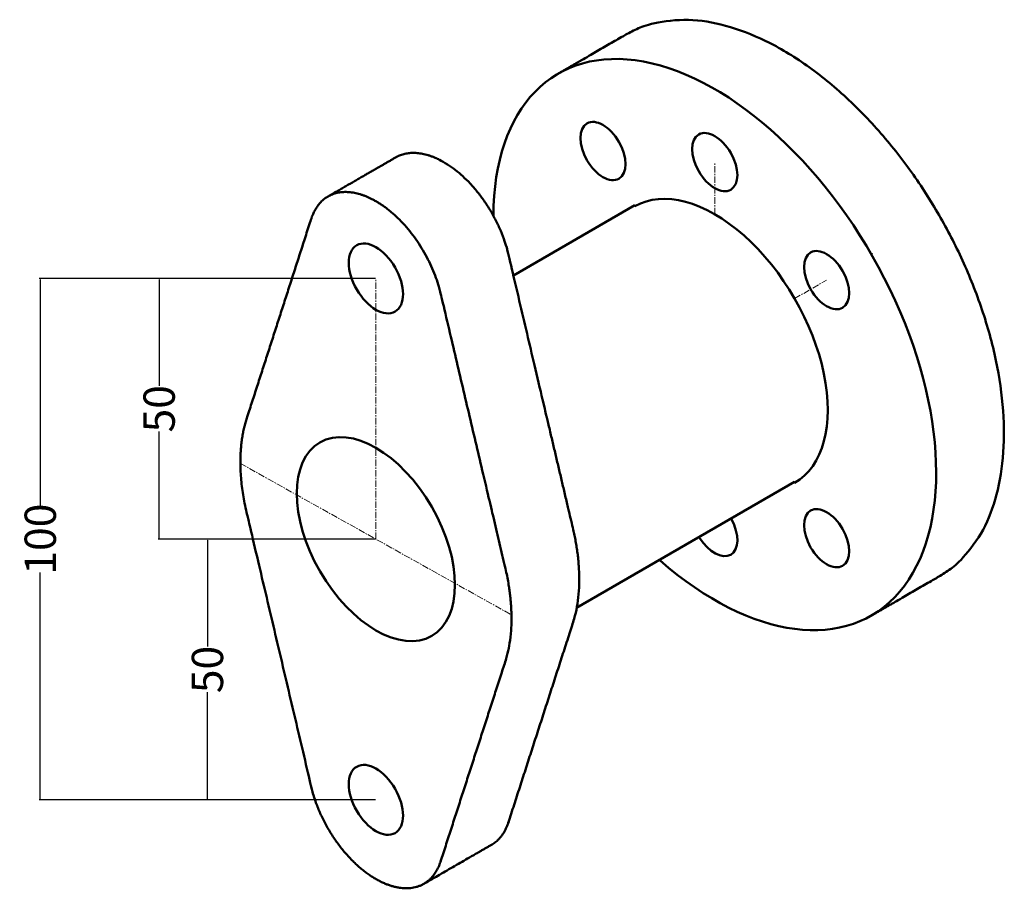
# Model space of a CAD drawing. Units: millimetres. Extents: x -79 to 109, y -50 to 116.
import ezdxf

# ---------------------------------------------------------------- set-up
doc = ezdxf.new("R2010")
doc.units = ezdxf.units.MM
doc.header["$MEASUREMENT"] = 0
doc.linetypes.add('CENTER', pattern=[2, 1.25, -0.25, 0.25, -0.25])
for name, color, linetype, lineweight in [('M-CNTR', 4, 'CENTER', 18), ('M-DIMS', 2, 'Continuous', 25), ('M-OUTL', 7, 'Continuous', 50)]:
    doc.layers.add(name, color=color, linetype=linetype, lineweight=lineweight)
doc.styles.get("Standard").update_dxf_attribs({"font": 'arial.ttf'})
doc.dimstyles.get("Standard").update_dxf_attribs({"dimtxt": 6, "dimasz": 0.18, "dimexe": 0.18, "dimexo": 0.0625, "dimgap": 0.09, "dimtad": 0, "dimtoh": 1, "dimdec": 0, "dimzin": 0, "dimdsep": 46, "dimtxsty": 'Standard', "dimcen": 0.09, "dimadec": 0, "dimazin": 0, "dimtfac": 1, "dimtdec": 0, "dimtofl": 0, "dimtmove": 0, "dimatfit": 3, "dimfxl": 1, "dimtolj": 1, "dimtzin": 0, "dimarcsym": 0})

# ---------------------------------------------------------------- blocks, each defined once
blk = doc.blocks.new('*D1')
at = {"layer": 'Defpoints', "color": 0, "transparency": 16777216}
for p in [(-11.21, 66.86), (-75.55, -33.14), (-11.21, -33.14)]:
    blk.add_point(p, dxfattribs=at)
at = {"layer": 'M-DIMS', "color": 0, "lineweight": -2, "transparency": 16777216}
for p, q in [((-11.27, 66.86), (-75.73, 66.86)), ((-75.55, 66.68), (-75.55, 23.29)), ((-75.55, -32.96), (-75.55, 10.44)), ((-11.27, -33.14), (-75.73, -33.14))]:
    blk.add_line(p, q, dxfattribs=at)
at = {"layer": 'M-DIMS', "color": 0, "transparency": 16777216}
for points in [[(-75.58, 66.68), (-75.52, 66.68), (-75.55, 66.86)], [(-75.58, -32.96), (-75.52, -32.96), (-75.55, -33.14)]]:
    blk.add_solid(points, dxfattribs=at)
at = {"layer": 'M-DIMS', "color": 0, "transparency": 16777216, "insert": (-75.55, 16.86), "char_height": 6, "attachment_point": 5, "rotation": 90}
blk.add_mtext('\\A1;100', dxfattribs=at)
blk = doc.blocks.new('*D2')
at = {"layer": 'Defpoints', "color": 0, "transparency": 16777216}
for p in [(-11.21, 66.86), (-52.76, 16.86), (-11.21, 16.86)]:
    blk.add_point(p, dxfattribs=at)
at = {"layer": 'M-DIMS', "color": 0, "lineweight": -2, "transparency": 16777216}
for p, q in [((-11.27, 66.86), (-52.94, 66.86)), ((-52.76, 66.68), (-52.76, 46.24)), ((-52.76, 17.04), (-52.76, 37.48)), ((-11.27, 16.86), (-52.94, 16.86))]:
    blk.add_line(p, q, dxfattribs=at)
at = {"layer": 'M-DIMS', "color": 0, "transparency": 16777216}
for points in [[(-52.79, 66.68), (-52.73, 66.68), (-52.76, 66.86)], [(-52.79, 17.04), (-52.73, 17.04), (-52.76, 16.86)]]:
    blk.add_solid(points, dxfattribs=at)
at = {"layer": 'M-DIMS', "color": 0, "transparency": 16777216, "insert": (-52.76, 41.86), "char_height": 6, "attachment_point": 5, "rotation": 90}
blk.add_mtext('\\A1;50', dxfattribs=at)
blk = doc.blocks.new('*D3')
at = {"layer": 'Defpoints', "color": 0, "transparency": 16777216}
for p in [(-11.21, 16.86), (-43.5, -33.14), (-11.21, -33.14)]:
    blk.add_point(p, dxfattribs=at)
at = {"layer": 'M-DIMS', "color": 0, "lineweight": -2, "transparency": 16777216}
for p, q in [((-11.27, 16.86), (-43.68, 16.86)), ((-43.5, 16.68), (-43.5, -3.76)), ((-43.5, -32.96), (-43.5, -12.52)), ((-11.27, -33.14), (-43.68, -33.14))]:
    blk.add_line(p, q, dxfattribs=at)
at = {"layer": 'M-DIMS', "color": 0, "transparency": 16777216}
for points in [[(-43.53, 16.68), (-43.47, 16.68), (-43.5, 16.86)], [(-43.53, -32.96), (-43.47, -32.96), (-43.5, -33.14)]]:
    blk.add_solid(points, dxfattribs=at)
at = {"layer": 'M-DIMS', "color": 0, "transparency": 16777216, "insert": (-43.5, -8.14), "char_height": 6, "attachment_point": 5, "rotation": 90}
blk.add_mtext('\\A1;50', dxfattribs=at)

msp = doc.modelspace()

# ---------------------------------------------------------------- linework, layer by layer
at = {"layer": 'M-CNTR'}
for p, q in [((53.74, 79.17), (53.74, 89.17)), ((83.75, 71.49), (84.05, 71.67)), ((-11.21, 16.86), (-11.21, 66.86)), ((69.05, 63), (75.18, 66.54)), ((-37.19, 31.38), (14.77, 2.34))]:
    msp.add_line(p, q, dxfattribs=at)
at = {"layer": 'M-OUTL'}
for p, q in [((-20.39, 82.58), (-20.39, 82.58)), ((-20.39, 82.58), (-20.39, 82.58)), ((15.17, 67.45), (38.43, 80.88)), ((27.24, 3.71), (69.05, 27.84)), ((14.19, -37.45), (14.19, -37.45))]:
    msp.add_line(p, q, dxfattribs=at)
for centre, major_axis, start_param, end_param in [((53.74, 54.17), (30.01, -51.97), 5.247811, 10.206143), ((53.74, 54.17), (15.31, -26.52), 6.283185, 9.424778), ((53.74, 19.17), (3.06, -5.3), 4.762663, 7.803708)]:
    msp.add_ellipse(centre, major_axis=major_axis, ratio=0.57735, start_param=start_param, end_param=end_param, dxfattribs=at)
for centre, major_axis in [((32.31, 91.29), (3.06, -5.3)), ((53.74, 89.17), (3.06, -5.3)), ((53.74, 89.17), (-3.06, 5.3)), ((-11.21, 66.86), (3.67, -6.36)), ((75.18, 66.54), (3.06, -5.3)), ((-11.21, 16.86), (10.72, -18.56)), ((75.18, 17.04), (3.06, -5.3)), ((-11.21, -33.14), (3.67, -6.36))]:
    msp.add_ellipse(centre, major_axis=major_axis, ratio=0.57735, dxfattribs=at)
for points, weights, knots in [([(83.75, 2.19), (90.25, 5.94), (96.74, 9.69), (126.75, 27.02), (96.74, 78.99), (66.73, 130.96), (36.73, 113.64), (30.23, 109.89), (23.74, 106.14)], [1, 1, 1, 0.707106781187, 1, 0.707106781187, 1, 1, 1], [0, 0, 0, 1, 1, 2.570796, 2.570796, 4.141593, 4.141593, 5.141593, 5.141593, 5.141593]), ([(14.18, -37.48), (20.37, -18.31), (26.57, 0.86), (29.02, 8.44), (26.57, 18.86), (20.37, 45.18), (14.18, 71.51), (11.98, 80.83), (4.88, 86.95), (-2.23, 93.06), (-7.4, 90.08), (-13.9, 86.33), (-20.39, 82.58)], [1, 1, 1, 0.953939196582, 1, 1, 1, 0.871298422885, 1, 0.871298422885, 1, 1, 1], [0, 0, 0, 1, 1, 1.609385, 1.609385, 2.609385, 2.609385, 3.635294, 3.635294, 4.661203, 4.661203, 5.661203, 5.661203, 5.661203]), ([(1.19, -44.98), (7.38, -25.81), (13.58, -6.64), (16.03, 0.94), (13.58, 11.36), (7.38, 37.68), (1.19, 64.01), (-1.67, 76.16), (-11.21, 81.67), (-20.74, 87.17), (-23.6, 78.32), (-29.67, 59.52), (-35.74, 40.72)], [1, 1, 1, 0.953939196582, 1, 1, 1, 0.806132343372, 1, 0.806132343372, 1, 1, 1], [0, 0, 0, 1, 1, 1.609385, 1.609385, 2.609385, 2.609385, 3.875805, 3.875805, 5.142224, 5.142224, 6.142224, 6.142224, 6.142224]), ([(-35.74, 40.72), (-38.58, 32.96), (-35.99, 21.97), (-29.86, -4.07), (-23.73, -30.1), (-21.09, -42.63), (-11.21, -48.33), (-1.32, -54.04), (1.31, -44.56)], [1, 0.949084922224, 1, 1, 1, 0.795752511379, 1, 0.795752511379, 1], [0, 0, 0, 0.640956, 0.640956, 1.640956, 1.640956, 2.942051, 2.942051, 4.243145, 4.243145, 4.243145]), ([(-1.88, -49.16), (-1.95, -49.2), (-2.02, -49.24), (4.47, -45.49), (10.97, -41.74), (13.39, -40.35), (14.3, -37.06)], [1, 1, 1, 1, 1, 0.966940942952, 1], [0, 0, 0, 1, 1, 2, 2, 2.515696, 2.515696, 2.515696])]:
    msp.add_rational_spline(points, weights, degree=2, knots=knots, dxfattribs=at)

# ---------------------------------------------------------------- dimensions: what is measured, and where the dimension line sits
at = {"layer": 'M-DIMS'}
for p1, p2, distance, picture, middle in [((-11.21, 66.86), (-11.21, -33.14), -64.34, '*D1', (-75.55, 16.86)), ((-11.21, 66.86), (-11.21, 16.86), -41.55, '*D2', (-52.76, 41.86)), ((-11.21, 16.86), (-11.21, -33.14), -32.29, '*D3', (-43.5, -8.14))]:
    dim = msp.add_aligned_dim(p1=p1, p2=p2, distance=distance, dimstyle='Standard', override={"dimclrd": 0, "dimclre": 0, "dimclrt": 0}, dxfattribs=at)
    dim.commit()
    dim.dimension.update_dxf_attribs({"geometry": picture, "text_midpoint": middle})

doc.saveas('drawing.dxf')
